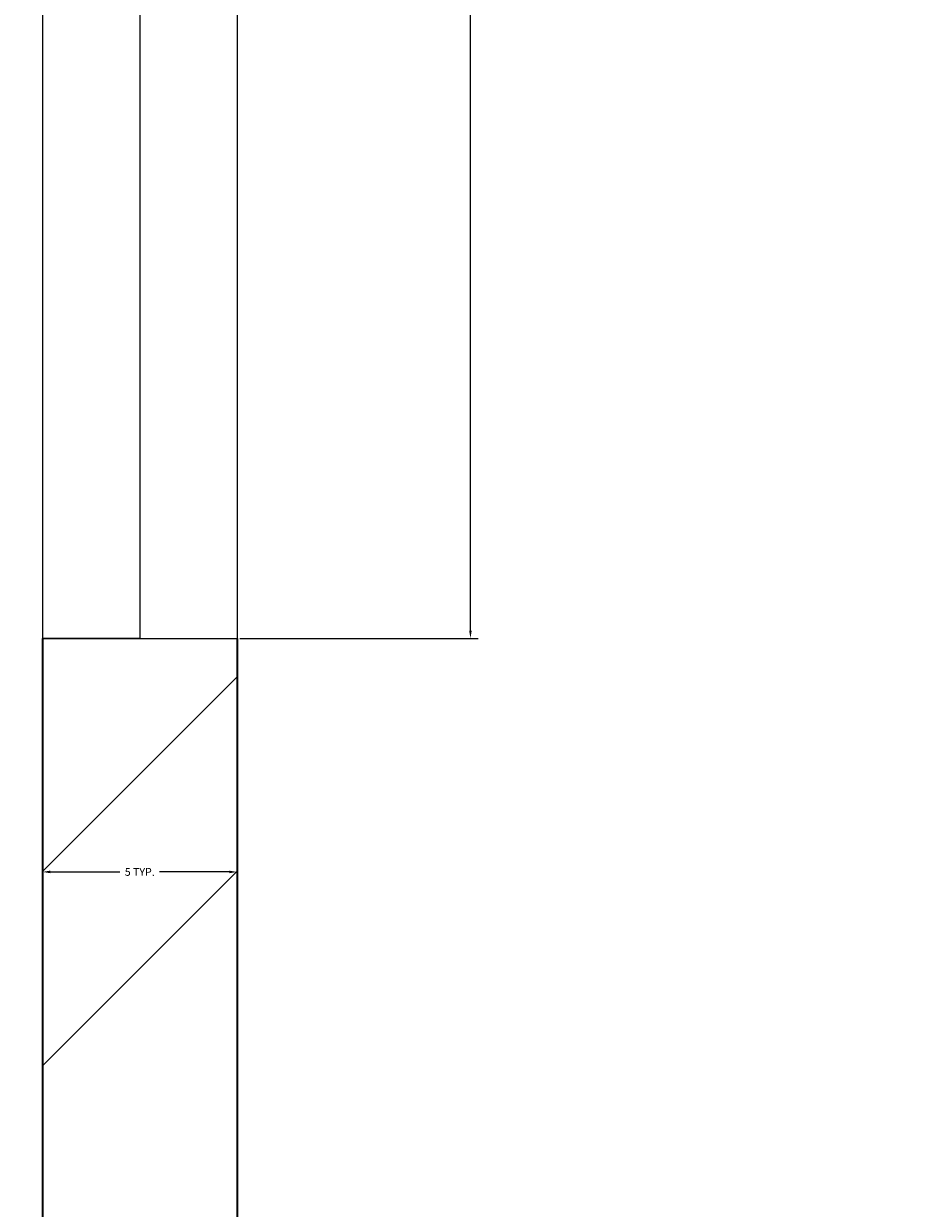
# Model space of a CAD drawing. Units: inches. Extents: x 1885 to 2748, y 783 to 2421.
# Tile 73 of 117: x 1992 to 2013, y 2093 to 2120. Entities that reach past the tile are written whole.
import ezdxf

# ---------------------------------------------------------------- set-up
doc = ezdxf.new("R2010")
doc.units = ezdxf.units.IN
for name, color, linetype, lineweight in [('A-ANNO-DIMS', 2, 'Continuous', 18), ('A-GLAZ', 181, 'Continuous', 18), ('A-WALL', 7, 'Continuous', 35)]:
    doc.layers.add(name, color=color, linetype=linetype, lineweight=lineweight)
doc.layers.add('A-WALL-PATT', color=85, linetype='Continuous', lineweight=13, true_color=0x58ba48)
doc.styles.get("Standard").update_dxf_attribs({"font": 'arial.ttf'})
doc.dimstyles.get("Standard").update_dxf_attribs({"dimtxt": 0.18, "dimasz": 0.18, "dimexe": 0.18, "dimexo": 0.0625, "dimgap": 0.09, "dimtad": 0, "dimtih": 1, "dimtoh": 1, "dimdec": 4, "dimzin": 0, "dimdsep": 46, "dimtxsty": 'Standard', "dimcen": 0.09, "dimadec": 0, "dimazin": 0, "dimtfac": 1, "dimtdec": 4, "dimtofl": 0, "dimtmove": 0, "dimatfit": 3, "dimfxl": 1, "dimtolj": 1, "dimtzin": 0, "dimarcsym": 0})

# ---------------------------------------------------------------- blocks, each defined once
blk = doc.blocks.new('WIN-36')
for p, q in [((0.004, 35.998), (0.004, -0.002)), ((2.254, 35.998), (2.254, -0.002)), ((4.504, 35.998), (4.504, -0.002)), ((2.254, -0.002), (0.004, -0.002)), ((0.004, -0.002), (4.504, -0.002))]:
    blk.add_line(p, q)
blk = doc.blocks.new('*D19')
at = {"layer": 'A-ANNO-DIMS', "color": 0, "lineweight": -2, "transparency": 16777216}
for p, q in [((1997.336, 2141.927), (2002.854, 2141.927)), ((2002.674, 2141.747), (2002.674, 2124.11)), ((2002.674, 2106.107), (2002.674, 2123.744)), ((1997.336, 2105.927), (2002.854, 2105.927))]:
    blk.add_line(p, q, dxfattribs=at)
at = {"layer": 'A-ANNO-DIMS', "color": 0, "transparency": 16777216}
for points in [[(2002.644, 2141.747), (2002.704, 2141.747), (2002.674, 2141.927)], [(2002.644, 2106.107), (2002.704, 2106.107), (2002.674, 2105.927)]]:
    blk.add_solid(points, dxfattribs=at)
at = {"layer": 'Defpoints', "color": 0, "transparency": 16777216}
for p in [(1997.274, 2141.927), (2002.674, 2141.927), (1997.274, 2105.927)]:
    blk.add_point(p, dxfattribs=at)
at = {"layer": 'A-ANNO-DIMS', "color": 0, "transparency": 16777216, "insert": (2002.674, 2123.927), "char_height": 0.18, "attachment_point": 5}
blk.add_mtext('\\A1;WINDOW 36 TYP.', dxfattribs=at)
blk = doc.blocks.new('*D20')
at = {"layer": 'A-ANNO-DIMS', "color": 0, "lineweight": -2, "transparency": 16777216}
for p, q in [((1992.774, 2105.864), (1992.774, 2100.347)), ((1997.274, 2105.864), (1997.274, 2100.347)), ((1992.954, 2100.527), (1994.565, 2100.527)), ((1997.094, 2100.527), (1995.482, 2100.527))]:
    blk.add_line(p, q, dxfattribs=at)
at = {"layer": 'A-ANNO-DIMS', "color": 0, "transparency": 16777216}
for points in [[(1992.954, 2100.557), (1992.954, 2100.497), (1992.774, 2100.527)], [(1997.094, 2100.557), (1997.094, 2100.497), (1997.274, 2100.527)]]:
    blk.add_solid(points, dxfattribs=at)
at = {"layer": 'Defpoints', "color": 0, "transparency": 16777216}
for p in [(1992.774, 2105.927), (1997.274, 2105.927), (1997.274, 2100.527)]:
    blk.add_point(p, dxfattribs=at)
at = {"layer": 'A-ANNO-DIMS', "color": 0, "transparency": 16777216, "insert": (1995.024, 2100.527), "char_height": 0.18, "attachment_point": 5}
blk.add_mtext('\\A1;5 TYP.', dxfattribs=at)
blk = doc.blocks.new('*D48')
at = {"layer": 'A-ANNO-DIMS', "color": 0, "lineweight": -2, "transparency": 16777216}
for p, q in [((1980.711, 2348.006), (1902.844, 2348.006)), ((1903.024, 2347.826), (1903.024, 2114.937)), ((1903.024, 1881.686), (1903.024, 2114.574)), ((2016.711, 1881.506), (1902.844, 1881.506))]:
    blk.add_line(p, q, dxfattribs=at)
at = {"layer": 'A-ANNO-DIMS', "color": 0, "transparency": 16777216}
for points in [[(1902.994, 2347.826), (1903.054, 2347.826), (1903.024, 2348.006)], [(1902.994, 1881.686), (1903.054, 1881.686), (1903.024, 1881.506)]]:
    blk.add_solid(points, dxfattribs=at)
at = {"layer": 'Defpoints', "color": 0, "transparency": 16777216}
for p in [(1903.024, 2348.006), (1980.774, 2348.006), (2016.774, 1881.506)]:
    blk.add_point(p, dxfattribs=at)
at = {"layer": 'A-ANNO-DIMS', "color": 0, "transparency": 16777216, "insert": (1903.024, 2114.756), "char_height": 0.18, "attachment_point": 5}
blk.add_mtext('\\A1;466.5', dxfattribs=at)

msp = doc.modelspace()

# ---------------------------------------------------------------- hatches: boundary and pattern name
at = {"layer": 'A-WALL-PATT'}
h = msp.add_hatch(dxfattribs=at)
h.set_pattern_fill('ANSI32', color=256)
h.paths.add_polyline_path([(2007.772, 2318.006), (1980.774, 2318.006), (1980.774, 2281.215), (1985.274, 2281.215), (1985.274, 2313.506), (2007.772, 2313.506), (2007.772, 2315.756)])
h.paths.add_polyline_path([(2094.324, 2318.006), (2067.772, 2318.006), (2067.772, 2313.506), (2094.324, 2313.506), (2094.324, 2315.756)])
h.paths.add_polyline_path([(2131.367, 2315.756), (2131.367, 2318.006), (2131.189, 2318.006), (2112.609, 2318.006), (2112.609, 2313.506), (2117.274, 2313.506), (2117.274, 2255.201), (2121.774, 2255.201), (2121.774, 2313.506), (2131.367, 2313.506)])
h.paths.add_polyline_path([(2190.512, 2318.006), (2155.367, 2318.006), (2155.367, 2313.506), (2169.774, 2313.506), (2169.774, 2229.506), (2121.774, 2229.506), (2121.774, 2233.451), (2119.524, 2233.451), (2117.274, 2233.451), (2117.274, 2201.101), (2121.774, 2201.101), (2121.774, 2225.006), (2169.774, 2225.006), (2169.774, 2165.006), (2306.274, 2165.006), (2306.274, 2066.006), (2310.774, 2066.006), (2344.274, 2066.006), (2486.274, 2066.006), (2486.274, 1886.006), (2483.02, 1886.006), (2483.02, 1881.506), (2486.274, 1881.506), (2486.274, 1880.678), (2490.774, 1880.678), (2490.774, 2070.506), (2344.274, 2070.506), (2310.774, 2070.506), (2310.774, 2165.006), (2310.774, 2173.636), (2308.524, 2173.636), (2306.274, 2173.636), (2306.274, 2169.506), (2174.274, 2169.506), (2174.274, 2313.506), (2190.512, 2313.506), (2190.512, 2315.756)])
h.paths.add_polyline_path([(1985.274, 2221.215), (1980.774, 2221.215), (1980.774, 2165.006), (1992.774, 2165.006), (1992.774, 2141.927), (1997.274, 2141.927), (1997.274, 2165.006), (2117.274, 2165.006), (2117.274, 2163.126), (2121.774, 2163.126), (2121.774, 2172.734), (2119.524, 2172.734), (2117.274, 2172.734), (2117.274, 2169.506), (1985.274, 2169.506)])
h.paths.add_polyline_path([(1997.274, 2105.927), (1992.774, 2105.927), (1992.774, 2070.506), (2016.774, 2070.506), (2016.774, 2059.123), (2019.024, 2059.123), (2021.274, 2059.123), (2021.274, 2070.506), (2117.274, 2070.506), (2117.274, 2022.506), (2114.423, 2022.506), (2114.423, 2018.006), (2123.627, 2018.006), (2123.627, 2020.256), (2123.627, 2022.506), (2121.774, 2022.506), (2121.774, 2142.587), (2119.524, 2142.587), (2117.274, 2142.587), (2117.274, 2075.006), (1997.274, 2075.006)])
h.paths.add_polyline_path([(2092.029, 2020.256), (2092.029, 2022.506), (2021.274, 2022.506), (2021.274, 2035.123), (2016.774, 2035.123), (2016.774, 2018.006), (2016.774, 1978.784), (2021.274, 1978.784), (2021.274, 2018.006), (2092.029, 2018.006)])
h.paths.add_polyline_path([(2260.938, 2022.506), (2153.105, 2022.506), (2153.105, 2020.256), (2153.105, 2018.006), (2155.274, 2018.006), (2155.274, 1886.006), (2107.629, 1886.006), (2107.629, 1881.506), (2182.911, 1881.506), (2182.911, 1883.756), (2182.911, 1886.006), (2159.774, 1886.006), (2159.774, 2018.006), (2260.938, 2018.006), (2260.938, 2020.256)])
h.paths.add_polyline_path([(2047.629, 1883.756), (2047.629, 1886.006), (2021.274, 1886.006), (2021.274, 1918.784), (2019.024, 1918.784), (2016.774, 1918.784), (2016.774, 1881.506), (2047.629, 1881.506)])
h.paths.add_polyline_path([(2306.361, 1883.756), (2306.361, 1886.006), (2296.274, 1886.006), (2296.274, 1982.006), (2316.535, 1982.006), (2316.535, 1984.256), (2316.535, 1986.506), (2296.274, 1986.506), (2296.274, 2022.506), (2289.276, 2022.506), (2289.276, 2018.006), (2291.774, 2018.006), (2291.774, 1886.006), (2242.911, 1886.006), (2242.911, 1881.506), (2306.361, 1881.506)], flags=17)
h.paths.add_polyline_path([(1985.274, 1843.006), (2021.6, 1843.006), (2021.534, 1845.441), (2021.477, 1847.506), (1980.774, 1847.506), (1980.774, 1809.446), (1985.274, 1809.446)])
h.paths.add_polyline_path([(2131.482, 1845.256), (2131.482, 1847.506), (2081.534, 1847.506), (2081.534, 1843.006), (2117.274, 1843.006), (2117.274, 1784.147), (2119.524, 1784.147), (2121.774, 1784.147), (2121.774, 1843.006), (2131.482, 1843.006)])
h.paths.add_polyline_path([(2203.886, 1847.506), (2155.482, 1847.506), (2155.482, 1843.006), (2169.774, 1843.006), (2169.774, 1759.006), (2121.774, 1759.006), (2121.774, 1761.457), (2117.274, 1761.457), (2117.274, 1730.429), (2121.774, 1730.429), (2121.774, 1754.506), (2177.421, 1754.506), (2177.421, 1756.756), (2177.421, 1759.006), (2174.274, 1759.006), (2174.274, 1843.006), (2203.886, 1843.006)])
h.paths.add_polyline_path([(2335.554, 1845.256), (2335.554, 1847.506), (2239.886, 1847.506), (2239.886, 1843.006), (2306.274, 1843.006), (2306.274, 1759.006), (2199.486, 1759.006), (2199.486, 1754.506), (2310.774, 1754.506), (2310.774, 1843.006), (2335.554, 1843.006)])
h.paths.add_polyline_path([(2348.774, 2022.506), (2344.274, 2022.506), (2344.274, 1986.506), (2341.681, 1986.506), (2341.681, 1982.006), (2344.274, 1982.006), (2344.274, 1886.006), (2330.361, 1886.006), (2330.361, 1881.506), (2361.627, 1881.506), (2361.627, 1883.756), (2361.627, 1886.006), (2348.774, 1886.006)], flags=17)
h.paths.add_polyline_path([(2283.251, 2315.756), (2283.251, 2318.006), (2238.512, 2318.006), (2238.512, 2313.506), (2283.251, 2313.506)], flags=17)
h.paths.add_polyline_path([(2363.274, 2348.006), (2388.677, 2348.006), (2388.677, 2350.256), (2388.677, 2352.506), (2358.774, 2352.506), (2358.774, 2348.006), (2358.774, 2318.006), (2344.481, 2318.006), (2344.481, 2313.506), (2358.774, 2313.506), (2358.774, 2229.506), (2310.774, 2229.506), (2310.774, 2231.952), (2306.274, 2231.952), (2306.274, 2205.611), (2310.774, 2205.611), (2310.774, 2225.006), (2358.774, 2225.006), (2358.774, 2211.506), (2452.329, 2211.506), (2452.329, 2213.756), (2452.329, 2216.006), (2363.274, 2216.006), (2363.274, 2318.006)])
h.paths.add_polyline_path([(2310.774, 2313.506), (2320.481, 2313.506), (2320.481, 2315.756), (2320.481, 2318.006), (2302.728, 2318.006), (2302.728, 2313.506), (2306.274, 2313.506), (2306.274, 2251.076), (2310.774, 2251.076)], flags=17)
h.paths.add_polyline_path([(2490.774, 2352.506), (2486.274, 2352.506), (2448.677, 2352.506), (2448.677, 2348.006), (2486.274, 2348.006), (2486.274, 2318.006), (2486.274, 2216.006), (2481.78, 2216.006), (2481.78, 2211.506), (2486.274, 2211.506), (2486.274, 2165.006), (2493.289, 2165.006), (2493.289, 2167.256), (2493.289, 2169.506), (2490.774, 2169.506), (2490.774, 2313.506), (2494.429, 2313.506), (2494.429, 2318.006), (2490.774, 2318.006)])
h.paths.add_polyline_path([(2534.653, 2318.006), (2515.691, 2318.006), (2515.691, 2313.506), (2534.653, 2313.506), (2534.653, 2315.756)])
h.paths.add_polyline_path([(2618.274, 2318.006), (2594.653, 2318.006), (2594.653, 2313.506), (2613.774, 2313.506), (2613.774, 2281.706), (2618.274, 2281.706)])
h.paths.add_polyline_path([(2618.274, 2221.706), (2613.774, 2221.706), (2613.774, 2169.506), (2554.019, 2169.506), (2554.019, 2165.006), (2613.774, 2165.006), (2613.774, 2152.878), (2618.274, 2152.878)])
h.paths.add_polyline_path([(2618.274, 2128.878), (2616.024, 2128.878), (2613.774, 2128.878), (2613.774, 2117.006), (2529.774, 2117.006), (2529.774, 2165.006), (2532.848, 2165.006), (2532.848, 2169.506), (2522.867, 2169.506), (2522.867, 2165.006), (2525.274, 2165.006), (2525.274, 2117.006), (2525.274, 2112.506), (2525.274, 2108.576), (2529.774, 2108.576), (2529.774, 2112.506), (2613.774, 2112.506), (2613.774, 2080.19), (2618.274, 2080.19)])
h.paths.add_polyline_path([(2618.274, 2044.19), (2616.024, 2044.19), (2613.774, 2044.19), (2613.774, 2015.506), (2529.774, 2015.506), (2529.774, 2088.582), (2527.524, 2088.582), (2525.274, 2088.582), (2525.274, 2011.006), (2613.774, 2011.006), (2613.774, 1956.755), (2618.274, 1956.755)])
h.paths.add_polyline_path([(2618.274, 1881.506), (2618.274, 1896.755), (2613.774, 1896.755), (2613.774, 1881.506), (2613.774, 1847.506), (2592.715, 1847.506), (2592.715, 1843.006), (2613.774, 1843.006), (2613.774, 1765.006), (2613.774, 1760.506), (2609.621, 1760.506), (2609.621, 1756.006), (2613.774, 1756.006), (2613.774, 1660.006), (2608.544, 1660.006), (2608.544, 1655.506), (2613.774, 1655.506), (2613.774, 1508.158), (2618.274, 1508.158)])
h.paths.add_polyline_path([(2565.774, 1843.006), (2568.997, 1843.006), (2568.997, 1847.506), (2490.774, 1847.506), (2490.774, 1849.7), (2488.524, 1849.7), (2486.274, 1849.7), (2486.274, 1847.506), (2477.274, 1847.506), (2477.274, 1838.506), (2477.274, 1821.493), (2486.274, 1821.493), (2486.274, 1838.506), (2561.274, 1838.506), (2561.274, 1765.006), (2486.274, 1765.006), (2486.274, 1786.157), (2477.274, 1786.157), (2477.274, 1765.006), (2477.274, 1756.006), (2486.274, 1756.006), (2565.774, 1756.006), (2585.621, 1756.006), (2585.621, 1758.256), (2585.621, 1760.506), (2565.774, 1760.506), (2565.774, 1765.006)])
h.paths.add_polyline_path([(2486.274, 1651.006), (2561.274, 1651.006), (2561.274, 1567.006), (2486.274, 1567.006), (2486.274, 1591.321), (2477.274, 1591.321), (2477.274, 1567.006), (2477.274, 1558.006), (2477.274, 1555.439), (2481.774, 1555.439), (2481.774, 1558.006), (2568.653, 1558.006), (2568.653, 1560.256), (2568.653, 1562.506), (2565.774, 1562.506), (2565.774, 1655.506), (2584.544, 1655.506), (2584.544, 1657.756), (2584.544, 1660.006), (2565.774, 1660.006), (2486.274, 1660.006), (2477.274, 1660.006), (2477.274, 1651.006), (2477.274, 1632.989), (2486.274, 1632.989)])
h.paths.add_polyline_path([(2449.967, 1883.756), (2449.967, 1886.006), (2421.627, 1886.006), (2421.627, 1881.506), (2449.967, 1881.506)], flags=17)
h.paths.add_polyline_path([(2447.274, 1847.506), (2395.554, 1847.506), (2395.554, 1843.006), (2442.774, 1843.006), (2442.774, 1809.27), (2447.274, 1809.27)])
h.paths.add_polyline_path([(1985.274, 1749.446), (1980.774, 1749.446), (1980.774, 1694.504), (1985.274, 1694.504), (1985.274, 1694.506), (1986.897, 1694.506), (1986.897, 1697.78), (1986.897, 1699.006), (1985.274, 1699.006)])
h.paths.add_polyline_path([(2152.774, 1699.006), (2121.774, 1699.006), (2121.774, 1703.668), (2119.524, 1703.668), (2117.274, 1703.668), (2117.274, 1699.006), (2009.219, 1699.006), (2009.219, 1694.506), (2148.274, 1694.506), (2148.274, 1692.631), (2152.774, 1692.631)])
h.paths.add_polyline_path([(2016.274, 1694.506), (2011.774, 1694.506), (2011.774, 1558.006), (2040.806, 1558.006), (2040.806, 1560.256), (2040.806, 1562.506), (2016.274, 1562.506)])
h.paths.add_polyline_path([(2152.774, 1663.017), (2150.524, 1663.017), (2148.274, 1663.017), (2148.274, 1562.506), (2100.806, 1562.506), (2100.806, 1558.006), (2165.119, 1558.006), (2165.119, 1560.256), (2165.119, 1562.506), (2152.774, 1562.506), (2152.774, 1610.506), (2224.774, 1610.506), (2224.774, 1607.99), (2229.274, 1607.99), (2229.274, 1615.006), (2152.774, 1615.006)])
h.paths.add_polyline_path([(2238.613, 1560.256), (2238.613, 1562.506), (2229.274, 1562.506), (2229.274, 1588.756), (2227.024, 1588.763), (2224.774, 1588.771), (2224.774, 1562.506), (2189.119, 1562.506), (2189.119, 1558.006), (2238.613, 1558.006)])
h.paths.add_polyline_path([(2336.024, 1560.256), (2336.024, 1562.506), (2310.774, 1562.506), (2310.774, 1656.347), (2308.524, 1656.347), (2306.274, 1656.347), (2306.274, 1562.506), (2286.613, 1562.506), (2286.613, 1558.006), (2336.024, 1558.006)])
h.paths.add_polyline_path([(2447.274, 1690.968), (2445.024, 1690.968), (2442.774, 1690.968), (2442.774, 1687.006), (2306.274, 1687.006), (2306.274, 1680.75), (2310.774, 1680.75), (2310.774, 1682.506), (2442.774, 1682.506), (2442.774, 1562.506), (2396.024, 1562.506), (2396.024, 1558.006), (2447.274, 1558.006)])
h.paths.add_polyline_path([(2447.274, 1749.27), (2445.024, 1749.27), (2442.774, 1749.27), (2442.774, 1717.232), (2447.274, 1717.232)])
h.paths.add_polyline_path([(2044.674, 1521.756), (2044.674, 1524.006), (2007.274, 1524.006), (2007.274, 1503.49), (2009.524, 1503.49), (2011.774, 1503.49), (2011.774, 1519.506), (2044.674, 1519.506)])
h.paths.add_polyline_path([(2177.969, 1521.756), (2177.969, 1524.006), (2104.674, 1524.006), (2104.674, 1519.506), (2145.774, 1519.506), (2145.774, 1387.506), (2143.37, 1387.506), (2143.37, 1383.006), (2251.585, 1383.006), (2251.585, 1385.256), (2251.585, 1387.506), (2150.274, 1387.506), (2150.274, 1519.506), (2177.969, 1519.506)])
h.paths.add_polyline_path([(2298.704, 1524.006), (2237.969, 1524.006), (2237.969, 1519.506), (2282.274, 1519.506), (2282.274, 1387.506), (2279.683, 1387.506), (2279.683, 1383.006), (2286.774, 1383.006), (2286.774, 1419.006), (2312.451, 1419.006), (2312.451, 1421.256), (2312.451, 1423.506), (2286.774, 1423.506), (2286.774, 1519.506), (2298.704, 1519.506), (2298.704, 1521.722)], flags=17)
h.paths.add_polyline_path([(2361.897, 1521.756), (2361.897, 1524.006), (2322.704, 1524.006), (2322.704, 1519.506), (2334.774, 1519.506), (2334.774, 1423.506), (2331.93, 1423.506), (2331.93, 1419.006), (2334.774, 1419.006), (2334.774, 1387.506), (2334.774, 1383.228), (2339.274, 1383.228), (2339.274, 1387.506), (2339.274, 1519.506), (2361.897, 1519.506)], flags=17)
h.paths.add_polyline_path([(2447.274, 1521.756), (2447.274, 1524.006), (2421.897, 1524.006), (2421.897, 1519.506), (2447.274, 1519.506)], flags=17)
h.paths.add_polyline_path([(2481.774, 1529.6), (2479.524, 1529.6), (2477.274, 1529.6), (2477.274, 1524.006), (2474.489, 1524.006), (2474.489, 1519.506), (2477.274, 1519.506), (2477.274, 1334.506), (2296.774, 1334.506), (2296.774, 1240.506), (2160.274, 1240.506), (2160.274, 1180.506), (2112.274, 1180.506), (2112.274, 1207.692), (2110.024, 1207.692), (2107.774, 1207.692), (2107.774, 1171.609), (2112.274, 1171.609), (2112.274, 1176.006), (2160.274, 1176.006), (2160.274, 1092.006), (2144.221, 1092.006), (2144.221, 1087.506), (2189.497, 1087.506), (2189.497, 1089.756), (2189.497, 1092.006), (2164.774, 1092.006), (2164.774, 1236.006), (2296.774, 1236.006), (2296.774, 1231.912), (2301.274, 1231.912), (2301.274, 1330.006), (2481.774, 1330.006), (2481.774, 1387.506)])
h.paths.add_polyline_path([(2618.274, 1448.158), (2613.774, 1448.158), (2613.774, 1382.506), (2529.774, 1382.506), (2525.274, 1382.506), (2525.274, 1307.062), (2529.774, 1307.062), (2529.774, 1378.006), (2613.774, 1378.006), (2613.774, 1354.988), (2618.274, 1354.988)])
h.paths.add_polyline_path([(2618.274, 1318.988), (2613.774, 1318.988), (2613.774, 1281.006), (2529.774, 1281.006), (2529.774, 1283.786), (2527.524, 1283.786), (2525.274, 1283.786), (2525.274, 1228.506), (2516.794, 1228.506), (2516.794, 1224.006), (2533.484, 1224.006), (2533.484, 1226.256), (2533.484, 1228.506), (2529.774, 1228.506), (2529.774, 1276.506), (2613.774, 1276.506), (2613.774, 1266.02), (2618.274, 1266.02)])
h.paths.add_polyline_path([(2618.274, 1134.964), (2613.774, 1134.964), (2613.774, 1092.006), (2594.545, 1092.006), (2594.545, 1087.506), (2618.274, 1087.506)])
h.paths.add_polyline_path([(2534.545, 1092.006), (2509.765, 1092.006), (2509.765, 1087.506), (2534.545, 1087.506), (2534.545, 1089.756)])
h.paths.add_polyline_path([(2481.274, 1224.006), (2484.117, 1224.006), (2484.117, 1226.256), (2484.117, 1228.506), (2476.774, 1228.506), (2476.774, 1198.506), (2471.61, 1198.506), (2471.61, 1194.006), (2476.774, 1194.006), (2476.774, 1062.006), (2436.894, 1062.006), (2436.894, 1057.506), (2476.774, 1057.506), (2481.274, 1057.506), (2481.274, 1062.006), (2481.274, 1087.506), (2485.354, 1087.506), (2485.354, 1089.756), (2485.354, 1092.006), (2481.274, 1092.006), (2481.274, 1117.506)])
h.paths.add_polyline_path([(2439.898, 1198.506), (2349.274, 1198.506), (2349.274, 1194.006), (2349.274, 1180.506), (2301.274, 1180.506), (2301.274, 1201.896), (2299.024, 1201.896), (2296.774, 1201.896), (2296.774, 1172.335), (2299.024, 1172.335), (2301.274, 1172.335), (2301.274, 1176.006), (2349.274, 1176.006), (2349.274, 1092.006), (2334.452, 1092.006), (2334.452, 1087.506), (2349.274, 1087.506), (2349.274, 1057.506), (2353.774, 1057.506), (2376.894, 1057.506), (2376.894, 1059.756), (2376.894, 1062.006), (2353.774, 1062.006), (2353.774, 1087.506), (2353.774, 1180.506), (2353.774, 1194.006), (2439.898, 1194.006), (2439.898, 1196.256)])
h.paths.add_polyline_path([(2270.596, 1089.756), (2270.596, 1092.006), (2249.497, 1092.006), (2249.497, 1087.506), (2270.596, 1087.506)], flags=17)
h.paths.add_polyline_path([(2310.452, 1092.006), (2301.274, 1092.006), (2301.274, 1153.292), (2296.774, 1153.292), (2296.774, 1092.006), (2293.786, 1092.006), (2293.786, 1087.506), (2310.452, 1087.506), (2310.452, 1089.756)], flags=17)
h.paths.add_polyline_path([(2112.274, 1150.328), (2110.024, 1150.328), (2107.774, 1150.328), (2107.774, 1092.006), (2104.465, 1092.006), (2104.465, 1087.506), (2120.221, 1087.506), (2120.221, 1089.756), (2120.221, 1092.006), (2112.274, 1092.006)])
h.paths.add_polyline_path([(2082.172, 1092.006), (2058.144, 1092.006), (2058.144, 1087.506), (2082.172, 1087.506), (2082.172, 1089.756)])
h.paths.add_polyline_path([(1975.774, 1145.638), (1971.274, 1145.638), (1971.274, 1087.506), (1980.774, 1087.506), (1998.144, 1087.506), (1998.144, 1089.756), (1998.144, 1092.006), (1985.274, 1092.006), (1975.774, 1092.006)])
h.paths.add_polyline_path([(2112.274, 1244.385), (2110.024, 1244.385), (2107.774, 1244.385), (2107.774, 1240.506), (1992.274, 1240.506), (1992.274, 1271.008), (1987.774, 1271.008), (1987.774, 1240.506), (1980.774, 1240.506), (1975.774, 1240.506), (1971.274, 1240.506), (1971.274, 1205.638), (1975.774, 1205.638), (1975.774, 1236.006), (2107.774, 1236.006), (2107.774, 1233.444), (2112.274, 1233.444), (2112.274, 1236.006)])
h.paths.add_polyline_path([(2112.274, 1383.006), (2114.783, 1383.006), (2114.783, 1385.256), (2114.783, 1387.506), (2102.476, 1387.506), (2102.476, 1383.006), (2107.774, 1383.006), (2107.774, 1335.006), (2011.774, 1335.006), (2011.774, 1349.939), (2007.274, 1349.939), (2007.274, 1335.006), (1987.774, 1335.006), (1987.774, 1330.506), (1987.774, 1307.008), (1992.274, 1307.008), (1992.274, 1330.506), (2007.274, 1330.506), (2107.774, 1330.506), (2107.774, 1264.711), (2112.274, 1264.711)])
h.paths.add_polyline_path([(2077.857, 1387.506), (2011.774, 1387.506), (2011.774, 1390.036), (2009.524, 1390.036), (2007.274, 1390.036), (2007.274, 1373.939), (2011.774, 1373.939), (2011.774, 1383.006), (2077.857, 1383.006)])
h.paths.add_polyline_path([(2011.774, 1443.49), (2007.274, 1443.49), (2007.274, 1410.248), (2011.774, 1410.248)])

# ---------------------------------------------------------------- linework, layer by layer
at = {"layer": 'A-WALL'}
for p, q in [((1992.774, 2105.927), (1992.774, 2070.506)), ((1997.274, 2105.927), (1997.274, 2075.006))]:
    msp.add_line(p, q, dxfattribs=at)

# ---------------------------------------------------------------- block references
at = {"layer": 'A-GLAZ'}
msp.add_blockref('WIN-36', (1992.77, 2105.929), dxfattribs=at)

# ---------------------------------------------------------------- dimensions: what is measured, and where the dimension line sits
at = {"layer": 'A-ANNO-DIMS'}
dim = msp.add_linear_dim(base=(1903.024, 2348.006), p1=(2016.774, 1881.506), p2=(1980.774, 2348.006), angle=90, dimstyle='Standard', override={"dimdec": 1, "dimlfac": 1, "dimrnd": 0, "dimzin": 0, "dimdsep": 46, "dimlunit": 2}, dxfattribs=at)
dim.commit()
dim.dimension.update_dxf_attribs({"geometry": '*D48', "text_midpoint": (1903.024, 2114.756)})
dim = msp.add_linear_dim(base=(2002.674, 2141.927), p1=(1997.274, 2105.927), p2=(1997.274, 2141.927), angle=90, text='WINDOW <> TYP.', dimstyle='Standard', override={"dimdec": 0, "dimlfac": 1, "dimrnd": 0, "dimzin": 0, "dimdsep": 46, "dimlunit": 2}, dxfattribs=at)
dim.commit()
dim.dimension.update_dxf_attribs({"geometry": '*D19', "text_midpoint": (2002.674, 2123.927)})
dim = msp.add_linear_dim(base=(1997.273597599, 2100.526836319), p1=(1992.773597599, 2105.926836319), p2=(1997.273597599, 2105.926836319), text='<> TYP.', dimstyle='Standard', override={"dimdec": 0, "dimlfac": 1, "dimrnd": 0, "dimzin": 0, "dimdsep": 46, "dimlunit": 2}, dxfattribs=at)
dim.commit()
dim.dimension.update_dxf_attribs({"geometry": '*D20', "text_midpoint": (1995.023597599, 2100.526836319)})

doc.saveas('drawing.dxf')
